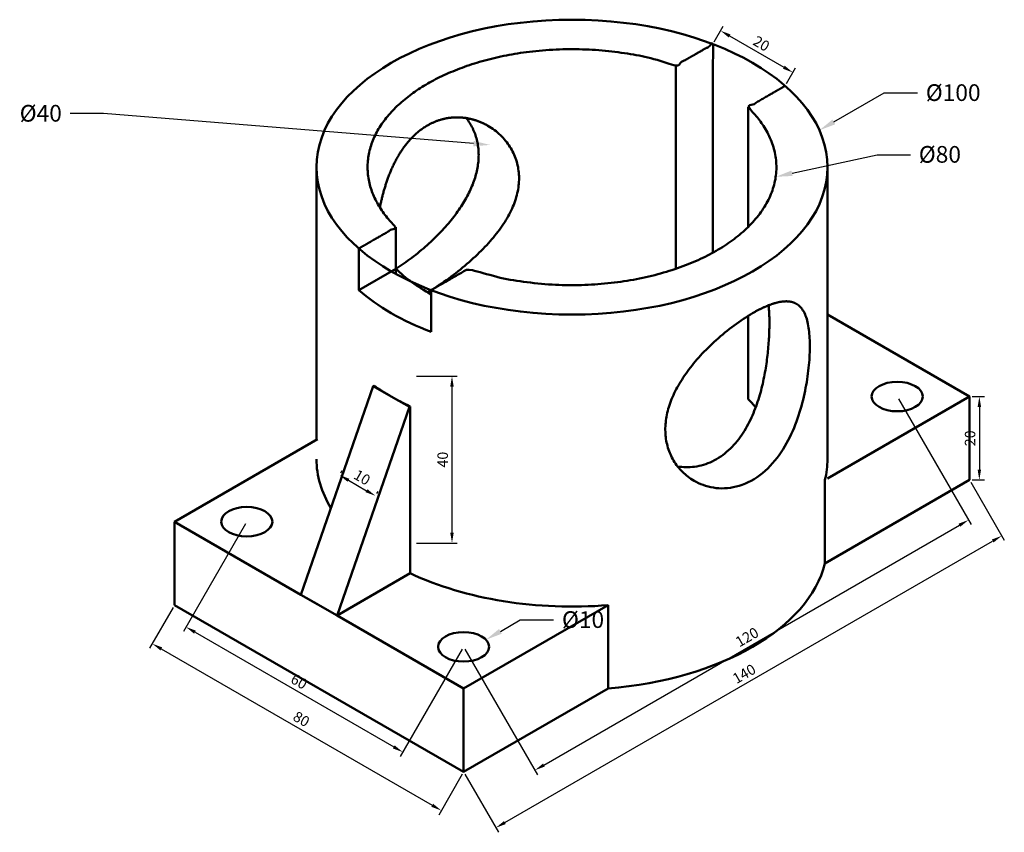
# Model space of a CAD drawing. Units: millimetres. Extents: x 2762 to 2998, y 1575 to 1770.
import ezdxf
from ezdxf import colors
from ezdxf.entities.mleader import LeaderData, LeaderLine
from ezdxf.math import Vec2, Vec3

# ---------------------------------------------------------------- set-up
doc = ezdxf.new("R2010")
doc.units = ezdxf.units.MM
for name, color, linetype, lineweight in [('M-DIMS', 2, 'Continuous', 25), ('M-OUTL', 7, 'Continuous', 50), ('M-TEXT', 3, 'Continuous', 25)]:
    doc.layers.add(name, color=color, linetype=linetype, lineweight=lineweight)
doc.styles.get("Standard").update_dxf_attribs({"font": 'arial.ttf'})
doc.dimstyles.new('ISO-25', dxfattribs={"dimtxt": 2.5, "dimasz": 2.5, "dimexe": 1.25, "dimexo": 0.625, "dimtad": 1, "dimtxsty": 'Standard', "dimcen": 2.5, "dimadec": 0, "dimazin": 0, "dimtfac": 1, "dimtmove": 0, "dimatfit": 3, "dimfxl": 1, "dimarcsym": 0})

# ---------------------------------------------------------------- blocks, each defined once
blk = doc.blocks.new('*D1')
at = {"layer": 'Defpoints', "color": 0, "transparency": 16777216}
for p in [(2989.2, 1659.81), (2996.93, 1646.43), (2867.96, 1589.81)]:
    blk.add_point(p, dxfattribs=at)
at = {"layer": 'M-DIMS', "color": 0, "lineweight": -2, "transparency": 16777216}
for p, q in [((2989.51, 1659.27), (2997.55, 1645.35)), ((2877.85, 1577.68), (2994.76, 1645.18)), ((2868.27, 1589.27), (2876.31, 1575.35))]:
    blk.add_line(p, q, dxfattribs=at)
at = {"layer": 'M-DIMS', "color": 0, "transparency": 16777216}
for points in [[(2994.56, 1645.54), (2994.97, 1644.82), (2996.93, 1646.43)], [(2877.64, 1578.04), (2878.06, 1577.32), (2875.68, 1576.43)]]:
    blk.add_solid(points, dxfattribs=at)
at = {"layer": 'M-DIMS', "color": 0, "transparency": 16777216, "insert": (2935.36, 1613.07), "char_height": 2.5, "attachment_point": 5, "rotation": 30}
blk.add_mtext('140', dxfattribs=at)
blk = doc.blocks.new('*D2')
at = {"layer": 'Defpoints', "color": 0, "transparency": 16777216}
for p in [(2971.88, 1679.81), (2988.97, 1650.22), (2867.96, 1619.81)]:
    blk.add_point(p, dxfattribs=at)
at = {"layer": 'M-DIMS', "color": 0, "lineweight": -2, "transparency": 16777216}
for p, q in [((2972.19, 1679.27), (2989.59, 1649.14)), ((2887.21, 1591.47), (2986.8, 1648.97)), ((2868.27, 1619.27), (2885.67, 1589.14))]:
    blk.add_line(p, q, dxfattribs=at)
at = {"layer": 'M-DIMS', "color": 0, "transparency": 16777216}
for points in [[(2986.59, 1649.33), (2987.01, 1648.61), (2988.97, 1650.22)], [(2887, 1591.83), (2887.42, 1591.11), (2885.04, 1590.22)]]:
    blk.add_solid(points, dxfattribs=at)
at = {"layer": 'M-DIMS', "color": 0, "transparency": 16777216, "insert": (2936.05, 1621.87), "char_height": 2.5, "attachment_point": 5, "rotation": 30}
blk.add_mtext('120', dxfattribs=at)
blk = doc.blocks.new('*D3')
at = {"layer": 'Defpoints', "color": 0, "transparency": 16777216}
for p in [(2798.68, 1629.81), (2867.96, 1589.81), (2862.62, 1580.57)]:
    blk.add_point(p, dxfattribs=at)
at = {"layer": 'M-DIMS', "color": 0, "lineweight": -2, "transparency": 16777216}
for p, q in [((2798.36, 1629.27), (2792.72, 1619.49)), ((2795.51, 1619.32), (2860.46, 1581.82)), ((2867.65, 1589.27), (2862, 1579.49))]:
    blk.add_line(p, q, dxfattribs=at)
at = {"layer": 'M-DIMS', "color": 0, "transparency": 16777216}
for points in [[(2795.71, 1619.68), (2795.3, 1618.96), (2793.34, 1620.57)], [(2860.67, 1582.18), (2860.25, 1581.46), (2862.62, 1580.57)]]:
    blk.add_solid(points, dxfattribs=at)
at = {"layer": 'M-DIMS', "color": 0, "transparency": 16777216, "insert": (2828.93, 1602.22), "char_height": 2.5, "attachment_point": 5, "rotation": 330}
blk.add_mtext('80', dxfattribs=at)
blk = doc.blocks.new('*D4')
at = {"layer": 'Defpoints', "color": 0, "transparency": 16777216}
for p in [(2816, 1649.81), (2867.96, 1619.81), (2853.39, 1594.57)]:
    blk.add_point(p, dxfattribs=at)
at = {"layer": 'M-DIMS', "color": 0, "lineweight": -2, "transparency": 16777216}
for p, q in [((2815.68, 1649.27), (2800.8, 1623.49)), ((2803.59, 1623.32), (2851.22, 1595.82)), ((2867.65, 1619.27), (2852.76, 1593.49))]:
    blk.add_line(p, q, dxfattribs=at)
at = {"layer": 'M-DIMS', "color": 0, "transparency": 16777216}
for points in [[(2803.8, 1623.69), (2803.38, 1622.96), (2801.43, 1624.57)], [(2851.43, 1596.19), (2851.01, 1595.46), (2853.39, 1594.57)]]:
    blk.add_solid(points, dxfattribs=at)
at = {"layer": 'M-DIMS', "color": 0, "transparency": 16777216, "insert": (2828.36, 1611.22), "char_height": 2.5, "attachment_point": 5, "rotation": 330}
blk.add_mtext('60', dxfattribs=at)
blk = doc.blocks.new('*D5')
at = {"layer": 'Defpoints', "color": 0, "transparency": 16777216}
for p in [(2838.2, 1661), (2846.86, 1656), (2846.86, 1656)]:
    blk.add_point(p, dxfattribs=at)
at = {"layer": 'M-DIMS', "color": 0, "lineweight": -2, "transparency": 16777216}
for p, q in [((2838.51, 1661.54), (2838.82, 1662.08)), ((2840.36, 1659.75), (2844.69, 1657.25)), ((2847.17, 1656.54), (2847.48, 1657.08))]:
    blk.add_line(p, q, dxfattribs=at)
at = {"layer": 'M-DIMS', "color": 0, "transparency": 16777216}
for points in [[(2840.57, 1660.11), (2840.15, 1659.39), (2838.2, 1661)], [(2844.9, 1657.61), (2844.48, 1656.89), (2846.86, 1656)]]:
    blk.add_solid(points, dxfattribs=at)
at = {"layer": 'M-DIMS', "color": 0, "transparency": 16777216, "insert": (2843.48, 1660.15), "char_height": 2.5, "attachment_point": 5, "rotation": 330}
blk.add_mtext('10', dxfattribs=at)
blk = doc.blocks.new('*D6')
at = {"layer": 'Defpoints', "color": 0, "transparency": 16777216}
for p in [(2856.07, 1684.69), (2856.07, 1644.69), (2865.18, 1644.69)]:
    blk.add_point(p, dxfattribs=at)
at = {"layer": 'M-DIMS', "color": 0, "lineweight": -2, "transparency": 16777216}
for p, q in [((2856.69, 1684.69), (2866.43, 1684.69)), ((2865.18, 1682.19), (2865.18, 1647.19)), ((2856.69, 1644.69), (2866.43, 1644.69))]:
    blk.add_line(p, q, dxfattribs=at)
at = {"layer": 'M-DIMS', "color": 0, "transparency": 16777216}
for points in [[(2864.76, 1682.19), (2865.59, 1682.19), (2865.18, 1684.69)], [(2864.76, 1647.19), (2865.59, 1647.19), (2865.18, 1644.69)]]:
    blk.add_solid(points, dxfattribs=at)
at = {"layer": 'M-DIMS', "color": 0, "transparency": 16777216, "insert": (2863.27, 1664.69), "char_height": 2.5, "attachment_point": 5, "rotation": 90}
blk.add_mtext('40', dxfattribs=at)
blk = doc.blocks.new('*D7')
at = {"layer": 'Defpoints', "color": 0, "transparency": 16777216}
for p in [(2927.71, 1764.31), (2946.88, 1757.51), (2945.03, 1754.31)]:
    blk.add_point(p, dxfattribs=at)
at = {"layer": 'M-DIMS', "color": 0, "lineweight": -2, "transparency": 16777216}
for p, q in [((2928.02, 1764.85), (2930.18, 1768.6)), ((2931.72, 1766.26), (2944.71, 1758.76)), ((2945.34, 1754.85), (2947.5, 1758.6))]:
    blk.add_line(p, q, dxfattribs=at)
at = {"layer": 'M-DIMS', "color": 0, "transparency": 16777216}
for points in [[(2931.93, 1766.63), (2931.51, 1765.9), (2929.56, 1767.51)], [(2944.92, 1759.13), (2944.51, 1758.4), (2946.88, 1757.51)]]:
    blk.add_solid(points, dxfattribs=at)
at = {"layer": 'M-DIMS', "color": 0, "transparency": 16777216, "insert": (2939.17, 1764.16), "char_height": 2.5, "attachment_point": 5, "rotation": 330}
blk.add_mtext('20', dxfattribs=at)
blk = doc.blocks.new('*D8')
at = {"layer": 'Defpoints', "color": 0, "transparency": 16777216}
for p in [(2989.2, 1679.81), (2989.2, 1659.81), (2991.57, 1659.81)]:
    blk.add_point(p, dxfattribs=at)
at = {"layer": 'M-DIMS', "color": 0, "lineweight": -2, "transparency": 16777216}
for p, q in [((2989.83, 1679.81), (2992.82, 1679.81)), ((2991.57, 1677.31), (2991.57, 1662.31)), ((2989.83, 1659.81), (2992.82, 1659.81))]:
    blk.add_line(p, q, dxfattribs=at)
at = {"layer": 'M-DIMS', "color": 0, "transparency": 16777216}
for points in [[(2991.16, 1677.31), (2991.99, 1677.31), (2991.57, 1679.81)], [(2991.16, 1662.31), (2991.99, 1662.31), (2991.57, 1659.81)]]:
    blk.add_solid(points, dxfattribs=at)
at = {"layer": 'M-DIMS', "color": 0, "transparency": 16777216, "insert": (2989.67, 1669.81), "char_height": 2.5, "attachment_point": 5, "rotation": 90}
blk.add_mtext('20', dxfattribs=at)

msp = doc.modelspace()

# ---------------------------------------------------------------- linework, layer by layer
at = {"layer": 'M-OUTL'}
for p, q in [((2918.82, 1759.176), (2918.82, 1710.446)), ((2936.14, 1749.176), (2936.14, 1720.446)), ((2955.176, 1664.814), (2955.176, 1734.814)), ((2851.738, 1720.446), (2851.738, 1709.191)), ((2842.852, 1705.32), (2842.852, 1715.32)), ((2842.852, 1705.32), (2851.738, 1710.449)), ((2860.173, 1695.32), (2860.173, 1705.32)), ((2936.14, 1679.179), (2936.14, 1699.156)), ((2828.987, 1632.314), (2846.308, 1682.314)), ((2846.308, 1682.314), (2846.525, 1682.44)), ((2850.638, 1679.814), (2846.308, 1682.314)), ((2854.968, 1677.314), (2850.638, 1679.814)), ((2989.202, 1659.814), (2989.202, 1679.814)), ((2837.647, 1627.314), (2854.968, 1677.314)), ((2854.968, 1677.314), (2855.185, 1677.44)), ((2855.185, 1637.44), (2855.185, 1677.44)), ((2954.561, 1639.814), (2989.202, 1659.814)), ((2954.561, 1639.814), (2954.561, 1659.814)), ((2828.987, 1632.314), (2798.676, 1649.814)), ((2798.676, 1629.814), (2798.676, 1649.814)), ((2855.185, 1637.44), (2837.647, 1627.314)), ((2833.317, 1629.811), (2828.987, 1632.311)), ((2828.987, 1632.311), (2837.647, 1627.311)), ((2867.958, 1589.814), (2798.676, 1629.814)), ((2867.958, 1609.814), (2902.599, 1629.814)), ((2902.599, 1609.814), (2902.599, 1629.814)), ((2867.958, 1609.814), (2837.647, 1627.314)), ((2867.958, 1589.814), (2902.599, 1609.814)), ((2867.958, 1609.811), (2867.958, 1589.811))]:
    msp.add_line(p, q, dxfattribs=at)
for points in [[(2868.6, 1746.579), (2868.822, 1746.288), (2869.035, 1745.992), (2869.24, 1745.692), (2869.436, 1745.386), (2869.624, 1745.076), (2869.804, 1744.761), (2869.975, 1744.443), (2870.138, 1744.12), (2870.292, 1743.792), (2870.437, 1743.461), (2870.574, 1743.127), (2870.702, 1742.788), (2870.822, 1742.446), (2870.932, 1742.101), (2871.034, 1741.752), (2871.128, 1741.4), (2871.212, 1741.044), (2871.288, 1740.686), (2871.355, 1740.325), (2871.413, 1739.961), (2871.462, 1739.594), (2871.502, 1739.224), (2871.533, 1738.853), (2871.556, 1738.479), (2871.569, 1738.102), (2871.573, 1737.724), (2871.569, 1737.343), (2871.555, 1736.961), (2871.533, 1736.577), (2871.501, 1736.191), (2871.461, 1735.803), (2871.412, 1735.414), (2871.354, 1735.023), (2871.287, 1734.631), (2871.211, 1734.238), (2871.126, 1733.844), (2871.033, 1733.448), (2870.93, 1733.052), (2870.819, 1732.654), (2870.7, 1732.256), (2870.572, 1731.856), (2870.435, 1731.456), (2870.289, 1731.055), (2870.135, 1730.653), (2869.972, 1730.251), (2869.801, 1729.847), (2869.621, 1729.443), (2869.433, 1729.039), (2869.236, 1728.634), (2869.031, 1728.228), (2868.818, 1727.822), (2868.596, 1727.416), (2868.366, 1727.009), (2868.128, 1726.602), (2867.882, 1726.195), (2867.627, 1725.787), (2867.365, 1725.379), (2867.094, 1724.972), (2866.815, 1724.564), (2866.529, 1724.156), (2866.234, 1723.748), (2865.932, 1723.341), (2865.622, 1722.933), (2865.304, 1722.526), (2864.979, 1722.12), (2864.646, 1721.713), (2864.305, 1721.307), (2863.956, 1720.902), (2863.601, 1720.497), (2863.237, 1720.092), (2862.866, 1719.688), (2862.488, 1719.285), (2862.102, 1718.883), (2861.71, 1718.482), (2861.31, 1718.082), (2860.903, 1717.684), (2860.49, 1717.287), (2860.07, 1716.892), (2859.643, 1716.5), (2859.21, 1716.109), (2858.771, 1715.721), (2858.327, 1715.335), (2857.877, 1714.953), (2857.421, 1714.575), (2856.962, 1714.2), (2856.497, 1713.83), (2856.029, 1713.464), (2855.558, 1713.104), (2855.083, 1712.749), (2854.606, 1712.4), (2854.127, 1712.058), (2853.648, 1711.724), (2853.168, 1711.397), (2852.69, 1711.08), (2852.213, 1710.772), (2851.738, 1710.473)], [(2859.298, 1744.814), (2859.456, 1744.905), (2859.616, 1744.993), (2859.775, 1745.079), (2859.936, 1745.163), (2860.096, 1745.244), (2860.258, 1745.324), (2860.42, 1745.401), (2860.582, 1745.476), (2860.745, 1745.549), (2860.908, 1745.62), (2861.072, 1745.688), (2861.236, 1745.755), (2861.4, 1745.819), (2861.565, 1745.881), (2861.729, 1745.941), (2861.894, 1745.998), (2862.06, 1746.054), (2862.225, 1746.107), (2862.39, 1746.158), (2862.556, 1746.206), (2862.722, 1746.253), (2862.887, 1746.297), (2863.053, 1746.34), (2863.218, 1746.38), (2863.384, 1746.418), (2863.549, 1746.453), (2863.714, 1746.487), (2863.879, 1746.519), (2864.044, 1746.548), (2864.208, 1746.575), (2864.372, 1746.601), (2864.536, 1746.624), (2864.699, 1746.645), (2864.863, 1746.664), (2865.025, 1746.682), (2865.188, 1746.697), (2865.35, 1746.71), (2865.512, 1746.721), (2865.673, 1746.731), (2865.834, 1746.738), (2865.994, 1746.744), (2866.154, 1746.748), (2866.313, 1746.75), (2866.472, 1746.75), (2866.631, 1746.748), (2866.789, 1746.745), (2866.946, 1746.74), (2867.103, 1746.733), (2867.259, 1746.724), (2867.414, 1746.714), (2867.569, 1746.702), (2867.723, 1746.689), (2867.877, 1746.673), (2868.03, 1746.657), (2868.182, 1746.638), (2868.334, 1746.618), (2868.485, 1746.597), (2868.635, 1746.574), (2868.785, 1746.549), (2868.934, 1746.523), (2869.082, 1746.495), (2869.229, 1746.466), (2869.376, 1746.436), (2869.522, 1746.404), (2869.667, 1746.371), (2869.812, 1746.336), (2869.956, 1746.3), (2870.099, 1746.263), (2870.241, 1746.224), (2870.383, 1746.184), (2870.524, 1746.143), (2870.664, 1746.101), (2870.803, 1746.057), (2870.942, 1746.012), (2871.079, 1745.965), (2871.216, 1745.918), (2871.352, 1745.869), (2871.487, 1745.819), (2871.622, 1745.768), (2871.756, 1745.716), (2871.889, 1745.663), (2872.021, 1745.609), (2872.152, 1745.553), (2872.282, 1745.496), (2872.412, 1745.439), (2872.541, 1745.38), (2872.669, 1745.32), (2872.796, 1745.259), (2872.922, 1745.197), (2873.048, 1745.134), (2873.172, 1745.07), (2873.296, 1745.005), (2873.419, 1744.939), (2873.541, 1744.873), (2873.662, 1744.805), (2873.783, 1744.736)], [(2847.898, 1725.149), (2847.943, 1725.371), (2847.989, 1725.594), (2848.035, 1725.817), (2848.083, 1726.041), (2848.132, 1726.264), (2848.182, 1726.488), (2848.233, 1726.713), (2848.285, 1726.937), (2848.338, 1727.162), (2848.392, 1727.387), (2848.447, 1727.612), (2848.504, 1727.838), (2848.561, 1728.064), (2848.62, 1728.29), (2848.68, 1728.516), (2848.741, 1728.742), (2848.803, 1728.969), (2848.867, 1729.195), (2848.932, 1729.422), (2848.998, 1729.649), (2849.066, 1729.876), (2849.134, 1730.103), (2849.205, 1730.33), (2849.276, 1730.557), (2849.349, 1730.784), (2849.423, 1731.011), (2849.499, 1731.238), (2849.576, 1731.465), (2849.655, 1731.692), (2849.735, 1731.919), (2849.817, 1732.146), (2849.9, 1732.372), (2849.984, 1732.599), (2850.071, 1732.825), (2850.159, 1733.051), (2850.248, 1733.277), (2850.339, 1733.502), (2850.432, 1733.727), (2850.526, 1733.952), (2850.623, 1734.177), (2850.72, 1734.401), (2850.82, 1734.625), (2850.921, 1734.848), (2851.025, 1735.071), (2851.13, 1735.294), (2851.237, 1735.516), (2851.346, 1735.737), (2851.456, 1735.958), (2851.569, 1736.178), (2851.684, 1736.398), (2851.8, 1736.617), (2851.919, 1736.835), (2852.04, 1737.052), (2852.162, 1737.269), (2852.287, 1737.485), (2852.414, 1737.699), (2852.543, 1737.913), (2852.674, 1738.126), (2852.808, 1738.338), (2852.943, 1738.548), (2853.081, 1738.758), (2853.221, 1738.966), (2853.363, 1739.173), (2853.508, 1739.379), (2853.654, 1739.583), (2853.804, 1739.785), (2853.955, 1739.987), (2854.108, 1740.186), (2854.264, 1740.384), (2854.422, 1740.58), (2854.583, 1740.774), (2854.746, 1740.967), (2854.911, 1741.157), (2855.078, 1741.345), (2855.248, 1741.532), (2855.42, 1741.716), (2855.595, 1741.898), (2855.772, 1742.078), (2855.951, 1742.255), (2856.132, 1742.429), (2856.315, 1742.601), (2856.501, 1742.771), (2856.689, 1742.937), (2856.878, 1743.101), (2857.07, 1743.262), (2857.264, 1743.419), (2857.459, 1743.574), (2857.657, 1743.725), (2857.856, 1743.873), (2858.057, 1744.018), (2858.26, 1744.16), (2858.465, 1744.298), (2858.671, 1744.432), (2858.878, 1744.563), (2859.087, 1744.691), (2859.298, 1744.814)], [(2873.783, 1744.736), (2874.194, 1744.49), (2874.595, 1744.233), (2874.986, 1743.966), (2875.365, 1743.688), (2875.735, 1743.401), (2876.093, 1743.105), (2876.44, 1742.8), (2876.777, 1742.486), (2877.102, 1742.165), (2877.416, 1741.835), (2877.719, 1741.497), (2878.01, 1741.152), (2878.289, 1740.8), (2878.557, 1740.442), (2878.813, 1740.076), (2879.057, 1739.704), (2879.289, 1739.327), (2879.508, 1738.943), (2879.715, 1738.554), (2879.91, 1738.159), (2880.092, 1737.759), (2880.261, 1737.355), (2880.417, 1736.946), (2880.561, 1736.532), (2880.691, 1736.114), (2880.808, 1735.692), (2880.912, 1735.266), (2881.002, 1734.837), (2881.079, 1734.404), (2881.142, 1733.968), (2881.192, 1733.529), (2881.228, 1733.088), (2881.251, 1732.644), (2881.259, 1732.197), (2881.254, 1731.749), (2881.236, 1731.298), (2881.204, 1730.846), (2881.158, 1730.393), (2881.098, 1729.938), (2881.025, 1729.482), (2880.939, 1729.025), (2880.839, 1728.566), (2880.726, 1728.107), (2880.599, 1727.647), (2880.46, 1727.187), (2880.307, 1726.726), (2880.142, 1726.264), (2879.964, 1725.802), (2879.773, 1725.34), (2879.569, 1724.878), (2879.353, 1724.415), (2879.125, 1723.953), (2878.885, 1723.491), (2878.633, 1723.029), (2878.369, 1722.568), (2878.093, 1722.107), (2877.806, 1721.646), (2877.507, 1721.185), (2877.197, 1720.724), (2876.875, 1720.264), (2876.543, 1719.804), (2876.199, 1719.344), (2875.845, 1718.885), (2875.479, 1718.426), (2875.103, 1717.967), (2874.716, 1717.509), (2874.319, 1717.051), (2873.912, 1716.594), (2873.494, 1716.137), (2873.066, 1715.681), (2872.628, 1715.225), (2872.179, 1714.77), (2871.721, 1714.316), (2871.254, 1713.862), (2870.777, 1713.41), (2870.29, 1712.959), (2869.794, 1712.509), (2869.289, 1712.061), (2868.776, 1711.614), (2868.254, 1711.17), (2867.724, 1710.729), (2867.187, 1710.29), (2866.642, 1709.854), (2866.091, 1709.422), (2865.534, 1708.995), (2864.972, 1708.573), (2864.406, 1708.157), (2863.836, 1707.747), (2863.263, 1707.344), (2862.689, 1706.95), (2862.115, 1706.565), (2861.543, 1706.19), (2860.974, 1705.827), (2860.409, 1705.476), (2859.85, 1705.138), (2859.298, 1704.814)], [(2941.057, 1701.691), (2941.092, 1701.356), (2941.124, 1701.013), (2941.152, 1700.663), (2941.177, 1700.305), (2941.198, 1699.938), (2941.216, 1699.565), (2941.231, 1699.184), (2941.243, 1698.795), (2941.252, 1698.4), (2941.257, 1697.997), (2941.259, 1697.587), (2941.259, 1697.17), (2941.255, 1696.747), (2941.247, 1696.318), (2941.237, 1695.882), (2941.224, 1695.44), (2941.207, 1694.993), (2941.187, 1694.539), (2941.163, 1694.08), (2941.137, 1693.615), (2941.107, 1693.145), (2941.073, 1692.669), (2941.036, 1692.189), (2940.995, 1691.704), (2940.951, 1691.214), (2940.903, 1690.719), (2940.851, 1690.221), (2940.795, 1689.718), (2940.734, 1689.212), (2940.67, 1688.702), (2940.601, 1688.188), (2940.528, 1687.671), (2940.45, 1687.152), (2940.367, 1686.629), (2940.28, 1686.104), (2940.187, 1685.576), (2940.09, 1685.046), (2939.986, 1684.513), (2939.878, 1683.978), (2939.763, 1683.442), (2939.642, 1682.903), (2939.516, 1682.363), (2939.382, 1681.822), (2939.242, 1681.279), (2939.096, 1680.736), (2938.942, 1680.191), (2938.78, 1679.647), (2938.611, 1679.101), (2938.434, 1678.556), (2938.249, 1678.011), (2938.055, 1677.467), (2937.853, 1676.923), (2937.641, 1676.38), (2937.42, 1675.839), (2937.189, 1675.299), (2936.948, 1674.762), (2936.696, 1674.227), (2936.434, 1673.695), (2936.16, 1673.166), (2935.875, 1672.642), (2935.578, 1672.123), (2935.269, 1671.608), (2934.948, 1671.1), (2934.613, 1670.599), (2934.266, 1670.105), (2933.905, 1669.619), (2933.532, 1669.143), (2933.145, 1668.677), (2932.745, 1668.222), (2932.331, 1667.78), (2931.903, 1667.351), (2931.464, 1666.936), (2931.011, 1666.538), (2930.548, 1666.156), (2930.073, 1665.793), (2929.588, 1665.448), (2929.093, 1665.124), (2928.589, 1664.82), (2928.078, 1664.537), (2927.561, 1664.276), (2927.038, 1664.038), (2926.512, 1663.823), (2925.982, 1663.63), (2925.451, 1663.46), (2924.919, 1663.313), (2924.388, 1663.188), (2923.859, 1663.085), (2923.332, 1663.004), (2922.808, 1662.943), (2922.287, 1662.903), (2921.771, 1662.882), (2921.26, 1662.88), (2920.755, 1662.897), (2920.256, 1662.931), (2919.763, 1662.982), (2919.278, 1663.05)], [(2947.72, 1702.048), (2947.988, 1701.879), (2948.242, 1701.69), (2948.481, 1701.482), (2948.707, 1701.255), (2948.919, 1701.01), (2949.118, 1700.748), (2949.305, 1700.467), (2949.48, 1700.17), (2949.643, 1699.856), (2949.796, 1699.525), (2949.937, 1699.178), (2950.068, 1698.815), (2950.189, 1698.437), (2950.3, 1698.043), (2950.402, 1697.634), (2950.494, 1697.21), (2950.577, 1696.772), (2950.651, 1696.319), (2950.717, 1695.852), (2950.774, 1695.371), (2950.823, 1694.876), (2950.864, 1694.367), (2950.896, 1693.845), (2950.92, 1693.31), (2950.936, 1692.763), (2950.945, 1692.203), (2950.945, 1691.631), (2950.937, 1691.048), (2950.921, 1690.454), (2950.898, 1689.849), (2950.866, 1689.233), (2950.826, 1688.607), (2950.777, 1687.972), (2950.721, 1687.327), (2950.656, 1686.673), (2950.582, 1686.011), (2950.499, 1685.341), (2950.407, 1684.662), (2950.307, 1683.976), (2950.196, 1683.283), (2950.076, 1682.583), (2949.945, 1681.876), (2949.805, 1681.163), (2949.653, 1680.445), (2949.49, 1679.721), (2949.316, 1678.993), (2949.13, 1678.26), (2948.931, 1677.524), (2948.72, 1676.785), (2948.495, 1676.043), (2948.257, 1675.299), (2948.004, 1674.555), (2947.736, 1673.809), (2947.453, 1673.063), (2947.153, 1672.318), (2946.836, 1671.574), (2946.502, 1670.833), (2946.149, 1670.094), (2945.777, 1669.36), (2945.385, 1668.631), (2944.973, 1667.909), (2944.54, 1667.196), (2944.084, 1666.492), (2943.606, 1665.8), (2943.106, 1665.122), (2942.582, 1664.46), (2942.036, 1663.816), (2941.466, 1663.193), (2940.873, 1662.592), (2940.259, 1662.018), (2939.624, 1661.473), (2938.97, 1660.959), (2938.299, 1660.48), (2937.613, 1660.036), (2936.914, 1659.631), (2936.204, 1659.265), (2935.488, 1658.941), (2934.766, 1658.657), (2934.043, 1658.416), (2933.321, 1658.216), (2932.603, 1658.057), (2931.891, 1657.938), (2931.186, 1657.857), (2930.49, 1657.813), (2929.804, 1657.805), (2929.131, 1657.831), (2928.471, 1657.89), (2927.825, 1657.979), (2927.194, 1658.097), (2926.578, 1658.243), (2925.977, 1658.415), (2925.393, 1658.612), (2924.826, 1658.832), (2924.275, 1659.075), (2923.741, 1659.339), (2923.225, 1659.622)], [(2937.24, 1699.814), (2937.397, 1699.904), (2937.552, 1699.993), (2937.707, 1700.08), (2937.862, 1700.165), (2938.015, 1700.25), (2938.168, 1700.332), (2938.32, 1700.414), (2938.471, 1700.494), (2938.622, 1700.573), (2938.772, 1700.65), (2938.921, 1700.726), (2939.069, 1700.8), (2939.216, 1700.873), (2939.362, 1700.944), (2939.508, 1701.014), (2939.652, 1701.083), (2939.796, 1701.15), (2939.938, 1701.215), (2940.08, 1701.279), (2940.22, 1701.342), (2940.36, 1701.403), (2940.499, 1701.462), (2940.636, 1701.52), (2940.772, 1701.576), (2940.908, 1701.631), (2941.042, 1701.685), (2941.175, 1701.737), (2941.307, 1701.787), (2941.438, 1701.836), (2941.568, 1701.884), (2941.696, 1701.929), (2941.824, 1701.974), (2941.95, 1702.017), (2942.075, 1702.058), (2942.199, 1702.098), (2942.322, 1702.136), (2942.443, 1702.173), (2942.564, 1702.209), (2942.683, 1702.243), (2942.801, 1702.276), (2942.918, 1702.307), (2943.034, 1702.336), (2943.149, 1702.365), (2943.262, 1702.392), (2943.374, 1702.417), (2943.486, 1702.441), (2943.596, 1702.464), (2943.705, 1702.485), (2943.813, 1702.505), (2943.919, 1702.524), (2944.025, 1702.541), (2944.129, 1702.557), (2944.233, 1702.571), (2944.335, 1702.584), (2944.436, 1702.596), (2944.536, 1702.607), (2944.635, 1702.616), (2944.732, 1702.624), (2944.829, 1702.63), (2944.925, 1702.636), (2945.019, 1702.64), (2945.113, 1702.643), (2945.205, 1702.644), (2945.297, 1702.645), (2945.387, 1702.644), (2945.477, 1702.641), (2945.565, 1702.638), (2945.652, 1702.634), (2945.739, 1702.628), (2945.824, 1702.621), (2945.908, 1702.613), (2945.992, 1702.603), (2946.074, 1702.593), (2946.156, 1702.581), (2946.236, 1702.569), (2946.316, 1702.555), (2946.394, 1702.54), (2946.472, 1702.524), (2946.549, 1702.506), (2946.625, 1702.488), (2946.699, 1702.468), (2946.774, 1702.448), (2946.847, 1702.426), (2946.919, 1702.403), (2946.99, 1702.38), (2947.061, 1702.355), (2947.13, 1702.329), (2947.199, 1702.302), (2947.267, 1702.274), (2947.334, 1702.245), (2947.4, 1702.214), (2947.466, 1702.183), (2947.531, 1702.151), (2947.594, 1702.118), (2947.657, 1702.084), (2947.72, 1702.048)], [(2923.225, 1659.622), (2922.836, 1659.855), (2922.457, 1660.099), (2922.09, 1660.354), (2921.732, 1660.619), (2921.386, 1660.894), (2921.05, 1661.178), (2920.725, 1661.472), (2920.411, 1661.774), (2920.108, 1662.085), (2919.817, 1662.403), (2919.536, 1662.73), (2919.267, 1663.064), (2919.009, 1663.405), (2918.762, 1663.753), (2918.527, 1664.107), (2918.304, 1664.468), (2918.092, 1664.835), (2917.891, 1665.208), (2917.703, 1665.587), (2917.526, 1665.971), (2917.361, 1666.361), (2917.207, 1666.756), (2917.066, 1667.155), (2916.936, 1667.559), (2916.819, 1667.968), (2916.713, 1668.382), (2916.619, 1668.799), (2916.538, 1669.221), (2916.468, 1669.647), (2916.411, 1670.076), (2916.366, 1670.509), (2916.334, 1670.945), (2916.313, 1671.384), (2916.305, 1671.826), (2916.309, 1672.271), (2916.325, 1672.719), (2916.354, 1673.169), (2916.395, 1673.621), (2916.448, 1674.076), (2916.513, 1674.533), (2916.59, 1674.991), (2916.68, 1675.451), (2916.781, 1675.913), (2916.895, 1676.377), (2917.02, 1676.841), (2917.158, 1677.307), (2917.307, 1677.775), (2917.468, 1678.243), (2917.641, 1678.712), (2917.826, 1679.183), (2918.022, 1679.655), (2918.23, 1680.127), (2918.45, 1680.6), (2918.681, 1681.074), (2918.924, 1681.549), (2919.178, 1682.024), (2919.443, 1682.5), (2919.72, 1682.977), (2920.008, 1683.453), (2920.307, 1683.93), (2920.617, 1684.407), (2920.938, 1684.885), (2921.27, 1685.362), (2921.613, 1685.839), (2921.967, 1686.316), (2922.331, 1686.793), (2922.706, 1687.269), (2923.091, 1687.745), (2923.487, 1688.22), (2923.893, 1688.695), (2924.31, 1689.169), (2924.737, 1689.642), (2925.174, 1690.114), (2925.621, 1690.585), (2926.078, 1691.055), (2926.544, 1691.523), (2927.02, 1691.989), (2927.506, 1692.453), (2928, 1692.914), (2928.503, 1693.372), (2929.015, 1693.827), (2929.534, 1694.279), (2930.061, 1694.726), (2930.595, 1695.168), (2931.135, 1695.604), (2931.681, 1696.035), (2932.232, 1696.458), (2932.787, 1696.874), (2933.346, 1697.282), (2933.906, 1697.68), (2934.467, 1698.067), (2935.028, 1698.443), (2935.586, 1698.807), (2936.142, 1699.157), (2936.694, 1699.493), (2937.24, 1699.814)], [(2955.176, 1699.456), (2989.202, 1679.811), (2955.176, 1660.166)], [(2798.676, 1649.811), (2832.955, 1669.601)]]:
    msp.add_lwpolyline(points, dxfattribs=at)
for centre, major_axis in [((2893.939, 1734.811), (-61.237, 0)), ((2971.881, 1679.811), (-6.124, 0)), ((2815.997, 1649.811), (-6.124, 0)), ((2867.958, 1619.811), (-6.124, 0))]:
    msp.add_ellipse(centre, major_axis=major_axis, ratio=0.5773503, dxfattribs=at)
for centre, major_axis, start_param, end_param in [((2893.939, 1724.814), (48.99, 0), 3.6743106, 3.9519374), ((2893.939, 1724.814), (61.237, 0), 3.7256329, 4.1283487), ((2893.939, 1704.814), (61.237, 0), 3.8268234, 3.9269908), ((2893.939, 1704.814), (61.237, 0), 3.9269908, 4.0271582), ((2893.939, 1664.814), (48.99, 0), 0.454059, 0.5327179), ((2893.939, 1664.814), (61.237, 0), 3.1415927, 3.4801443), ((2893.939, 1664.814), (61.237, 0), 6.1412883, 6.2831853), ((2893.939, 1644.814), (61.237, 0), 4.854286, 6.1412883), ((2893.939, 1664.814), (61.237, 0), 4.0271582, 4.854286)]:
    msp.add_ellipse(centre, major_axis=major_axis, ratio=0.5773503, start_param=start_param, end_param=end_param, dxfattribs=at)
for points, weights, knots in [([(2927.705, 1714.318), (2927.705, 1739.312), (2927.705, 1764.306), (2923.262, 1761.741), (2918.82, 1759.176), (2886.131, 1770.303), (2859.298, 1754.811), (2832.465, 1739.319), (2851.738, 1720.446), (2847.295, 1717.881), (2842.852, 1715.316)], [1, 1, 1, 1, 1, 0.790569415042, 1, 0.790569415042, 1, 1, 1], [0, 0, 0, 1, 1, 2, 2, 3.3181161, 3.3181161, 4.6362321, 4.6362321, 5.6362321, 5.6362321, 5.6362321]), ([(2860.173, 1705.316), (2864.616, 1707.881), (2869.058, 1710.446), (2901.747, 1699.319), (2928.58, 1714.811), (2955.413, 1730.303), (2936.14, 1749.176), (2940.583, 1751.741), (2945.026, 1754.306)], [1, 1, 1, 0.790569415042, 1, 0.790569415042, 1, 1, 1], [0, 0, 0, 1, 1, 2.3181161, 2.3181161, 3.6362321, 3.6362321, 4.6362321, 4.6362321, 4.6362321])]:
    msp.add_rational_spline(points, weights, degree=2, knots=knots, dxfattribs=at)
msp.add_open_spline([(2832.702, 1734.811), (2832.702, 1702.133), (2832.702, 1669.456)], degree=2, dxfattribs=at)

# ---------------------------------------------------------------- dimensions: what is measured, and where the dimension line sits
at = {"layer": 'M-DIMS'}
for p1, p2, distance, picture, middle in [((2927.705, 1764.306), (2945.026, 1754.306), 3.705, '*D7', (2939.169, 1764.161)), ((2856.068, 1684.691), (2856.068, 1644.691), 9.108, '*D6', (2863.274, 1664.691)), ((2867.958, 1619.811), (2971.881, 1679.811), -34.17, '*D2', (2936.054, 1621.865)), ((2989.202, 1679.811), (2989.202, 1659.811), 2.37, '*D8', (2989.671, 1669.811)), ((2838.197, 1661.001), (2846.858, 1656.001), 0, '*D5', (2843.478, 1660.148)), ((2867.958, 1589.811), (2989.202, 1659.811), -15.453, '*D1', (2935.356, 1613.074)), ((2815.997, 1649.811), (2867.958, 1619.811), -29.141, '*D4', (2828.358, 1611.221)), ((2798.676, 1629.811), (2867.958, 1589.811), -10.67, '*D3', (2828.933, 1602.217))]:
    dim = msp.add_aligned_dim(p1=p1, p2=p2, distance=distance, dimstyle='ISO-25', override={"dimclrd": 0, "dimclre": 0, "dimclrt": 0}, dxfattribs=at)
    dim.commit()
    dim.dimension.update_dxf_attribs({"geometry": picture, "text_midpoint": middle})

# ---------------------------------------------------------------- leaders
at = {"layer": 'M-TEXT'}
ml = msp.add_multileader_mtext('Standard', dxfattribs=at)
ml.set_content('%%C100', color=256)
ml.set_leader_properties()
ml.build(insert=Vec2(0, 0))
ctx = ml.context
ctx.base_point, ctx.plane_origin = Vec3(2976.734, 1752.601), Vec3(2953.231, 1743.651)
notes = []
notes.append((ctx, [(0, (1, 1, 0), (2968.734, 1752.601), (1, 0), 8, [(0, [(2953.231, 1743.651)], 0, [])])]))
ctx.mtext.insert, ctx.mtext.flow_direction = Vec3(2978.734, 1754.681), 5
ml = msp.add_multileader_mtext('Standard', dxfattribs=at)
ml.set_content('%%C40', color=256)
ml.set_leader_properties()
ml.build(insert=Vec2(0, 0))
ctx = ml.context
ctx.base_point, ctx.plane_origin = Vec3(2759.609, 1747.649), Vec3(2874.328, 1740.144)
ctx.text_align_type = 2
notes.append((ctx, [(0, (1, 1, 0), (2781.677, 1747.649), (-1, 0), 8, [(0, [(2874.328, 1740.144)], 0, [])])]))
ctx.mtext.insert, ctx.mtext.alignment, ctx.mtext.flow_direction = Vec3(2771.677, 1749.729), 3, 5
ml = msp.add_multileader_mtext('Standard', dxfattribs=at)
ml.set_content('%%C80', color=256)
ml.set_leader_properties()
ml.build(insert=Vec2(0, 0))
ctx = ml.context
ctx.base_point, ctx.plane_origin = Vec3(2975.06, 1737.797), Vec3(2942.764, 1732.495)
notes.append((ctx, [(0, (1, 1, 0), (2967.06, 1737.797), (1, 0), 8, [(0, [(2942.764, 1732.495)], 0, [])])]))
ctx.mtext.insert, ctx.mtext.flow_direction = Vec3(2977.06, 1739.878), 5
ml = msp.add_multileader_mtext('Standard', dxfattribs=at)
ml.set_content('%%C10', color=256)
ml.set_leader_properties()
ml.build(insert=Vec2(0, 0))
ctx = ml.context
ctx.base_point, ctx.plane_origin = Vec3(2889.537, 1626.262), Vec3(2873.321, 1621.518)
notes.append((ctx, [(0, (1, 1, 0), (2881.537, 1626.262), (1, 0), 8, [(0, [(2873.321, 1621.518)], 0, [])])]))
ctx.mtext.insert, ctx.mtext.flow_direction = Vec3(2891.537, 1628.342), 5
for ctx, leaders in notes:
    for number, flags, end, landing, length, lines in leaders:
        leader = LeaderData()
        leader.index, (leader.has_last_leader_line, leader.has_dogleg_vector, leader.attachment_direction) = number, flags
        leader.last_leader_point, leader.dogleg_vector, leader.dogleg_length = Vec3(end), Vec3(landing), length
        for number, points, colour, breaks in lines:
            line = LeaderLine()
            line.index, line.vertices, line.color, line.breaks = number, Vec3.list(points), colors.encode_raw_color(colour), breaks
            leader.lines.append(line)
        ctx.leaders.append(leader)

doc.saveas('drawing.dxf')
